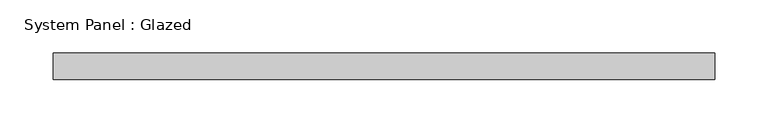
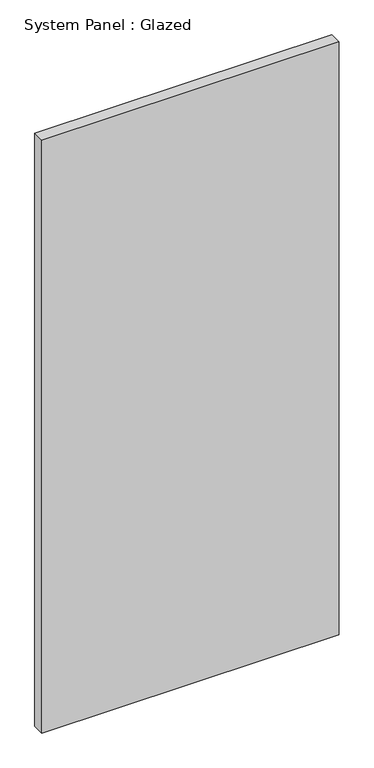
"""IFC4 building model written with IfcOpenShell, lengths in millimetres: plate geometry, System Panel : Glazed."""

from ifc_helpers import new_model, si_unit, origin, origin_with_axes, place, context, project, spatial, polyline, outline, extrude, source, transform, mapped, element, save


def system_panel_glazed_68555a4f(model_context):
    return source(origin(), model_context, "Body", "SweptSolid", [
        extrude(outline(polyline([(312.2083333, 19.05), (-312.2083333, 19.05), (-312.2083333, 44.45), (312.2083333, 44.45), (312.2083333, 19.05)])), origin_with_axes(), (0.0, 0.0, 1.0), 1315.3193903),
    ])


if __name__ == "__main__":
    model = new_model("IFC4")
    model_context = context("Model", 3, world=origin())
    ifc_project = project(units=[si_unit("LENGTHUNIT", "METRE", prefix="MILLI")], contexts=[model_context])
    site = spatial("IfcSite", under=ifc_project)
    building = spatial("IfcBuilding", under=site)
    placement = place(None, origin())
    system_panel_glazed_shape = system_panel_glazed_68555a4f(model_context)
    element("IfcPlate", 1, ObjectType="System Panel : Glazed", at=placement, inside=building, context=model_context, shape_type="MappedRepresentation", body=[
        mapped(system_panel_glazed_shape, transform((0.0, 0.0, 0.0), x_axis=(1.0, 0.0, 0.0), y_axis=(0.0, 1.0, 0.0), z_axis=(0.0, 0.0, 1.0))),
    ])
    save(model, "model.ifc")

# Revit data of these elements
# Type "System Panel : Glazed"
#   Construction Type Id = "GSP4R"
#   Analytic Construction = "1/8 in Pilkington single glazing"
#   Visual Light Transmittance = 0.9
#   Solar Heat Gain Coefficient = 0.86
#   Heat Transfer Coefficient (U) = 1.18115 BTU/(h·ft²·°F)
#   Define Thermal Properties by = 1
# Element 1 (IfcPlate, "System Panel : Glazed")
#   Materials on its faces: "Glass"
# Materials
#   "Glass": class "Glass", colour RGB 0 128 192, transparency 0.75, Description = "Soda Lime Glass", Cost = 0
